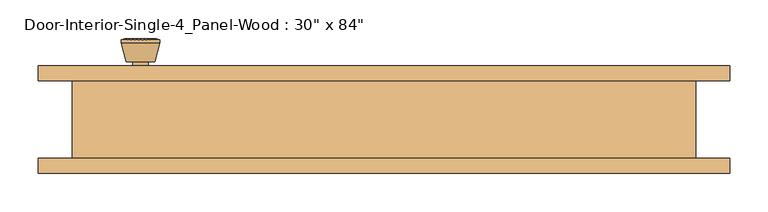
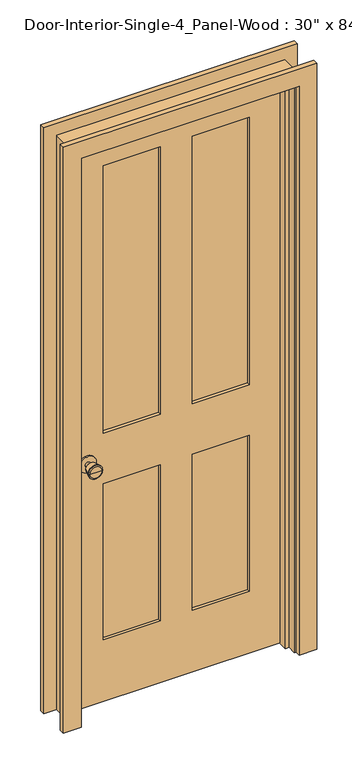
"""IFC4 building model written with IfcOpenShell, lengths in millimetres: door geometry."""

from ifc_helpers import new_model, si_unit, point, frame, frame_2d, origin, place, context, project, spatial, polyline, circle_curve, trimmed, segment, composite_curve, outline, extrude, faceted_brep, source, transform, mapped, element, save
from ifc_brep_helpers import plane_surface, cylinder_surface, revolved_surface, advanced_brep


def door_bd7b73b2(model_context):
    return source(origin(), model_context, "Body", "SolidModel", [
        advanced_brep(
        [(-317.5, 6.7, 914.4), (-307.5, 6.7, 914.4), (-327.5, 6.7, 914.4), (-297.0241324, -42.3, 914.4), (-317.5, -42.3, 914.4), (-337.9758676, -42.3, 914.4), (-292.5, -40.4721319, 914.4), (-342.5, -40.4721319, 914.4), (-292.5, -37.0084537, 914.4), (-342.5, -37.0084537, 914.4), (-298.863764, -12.3, 914.4), (-336.136236, -12.3, 914.4), (-307.5, -12.3, 914.4), (-327.5, -12.3, 914.4)],
        [
            (0, 1),
            (1, 2, circle_curve(frame((-317.5, 6.7, 914.4), z_axis=(0.0, 1.0, 0.0), x_axis=(-1.0, 0.0, 0.0)), 10.0)),
            (2, 0),
            (2, 1, circle_curve(frame((-317.5, 6.7, 914.4), z_axis=(0.0, 1.0, 0.0), x_axis=(-1.0, 0.0, 0.0)), 10.0)),
            (3, 4),
            (4, 5),
            (5, 3, circle_curve(frame((-317.5, -42.3, 914.4), z_axis=(0.0, -1.0, 0.0), x_axis=(-1.0, 0.0, 0.0)), 20.4758676)),
            (3, 5, circle_curve(frame((-317.5, -42.3, 914.4), z_axis=(0.0, -1.0, 0.0), x_axis=(-1.0, 0.0, 0.0)), 20.4758676)),
            (6, 3),
            (5, 7),
            (7, 6, circle_curve(frame((-317.5, -40.4721319, 914.4), z_axis=(0.0, -1.0, 0.0), x_axis=(-1.0, 0.0, 0.0)), 25.0)),
            (6, 7, circle_curve(frame((-317.5, -40.4721319, 914.4), z_axis=(0.0, -1.0, 0.0), x_axis=(-1.0, 0.0, 0.0)), 25.0)),
            (8, 6),
            (7, 9),
            (9, 8, circle_curve(frame((-317.5, -37.0084537, 914.4), z_axis=(0.0, -1.0, 0.0), x_axis=(-1.0, 0.0, 0.0)), 25.0)),
            (8, 9, circle_curve(frame((-317.5, -37.0084537, 914.4), z_axis=(0.0, -1.0, 0.0), x_axis=(-1.0, 0.0, 0.0)), 25.0)),
            (10, 8),
            (9, 11),
            (11, 10, circle_curve(frame((-317.5, -12.3, 914.4), z_axis=(0.0, -1.0, 0.0), x_axis=(-1.0, 0.0, 0.0)), 18.636236)),
            (10, 11, circle_curve(frame((-317.5, -12.3, 914.4), z_axis=(0.0, -1.0, 0.0), x_axis=(-1.0, 0.0, 0.0)), 18.636236)),
            (12, 10),
            (11, 13),
            (13, 12, circle_curve(frame((-317.5, -12.3, 914.4), z_axis=(0.0, -1.0, 0.0), x_axis=(-1.0, 0.0, 0.0)), 10.0)),
            (12, 13, circle_curve(frame((-317.5, -12.3, 914.4), z_axis=(0.0, -1.0, 0.0), x_axis=(-1.0, 0.0, 0.0)), 10.0)),
            (1, 12),
            (13, 2),
        ],
        [
            plane_surface(frame((-317.5, 6.7, 914.4), z_axis=(0.0, 1.0, 0.0), x_axis=(-1.0, 0.0, 0.0))),
            plane_surface(frame((-317.5, -42.3, 914.4), z_axis=(0.0, -1.0, 0.0), x_axis=(-1.0, 0.0, 0.0))),
            revolved_surface(polyline([(-337.9758676, -42.3, 914.4), (-342.5, -40.4721319, 914.4)]), (-317.5, 6.7, 914.4), (0.0, 1.0, 0.0)),
            cylinder_surface(frame((-317.5, 6.7, 914.4), z_axis=(0.0, 1.0, 0.0), x_axis=(-1.0, 0.0, 0.0)), 25.0),
            revolved_surface(polyline([(-342.5, -37.0084537, 914.4), (-336.136236, -12.3, 914.4)]), (-317.5, 6.7, 914.4), (0.0, 1.0, 0.0)),
            plane_surface(frame((-317.5, -12.3, 914.4), z_axis=(0.0, 1.0, 0.0), x_axis=(-1.0, 0.0, 0.0))),
            cylinder_surface(frame((-317.5, 6.7, 914.4), z_axis=(0.0, 1.0, 0.0), x_axis=(-1.0, 0.0, 0.0)), 10.0),
        ],
        [
            (0, [[1, 2, 3]]),
            (0, [[-3, 4, -1]]),
            (1, [[5, 6, 7]]),
            (1, [[-6, -5, 8]]),
            (2, [[9, -7, 10, 11]]),
            (2, [[-10, -8, -9, 12]]),
            (3, [[13, -11, 14, 15]]),
            (3, [[-14, -12, -13, 16]]),
            (4, [[17, -15, 18, 19]]),
            (4, [[-18, -16, -17, 20]]),
            (5, [[21, -19, 22, 23]]),
            (5, [[-22, -20, -21, 24]]),
            (6, [[25, -23, 26, -2]]),
            (6, [[-26, -24, -25, -4]]),
        ],
    ),
        extrude(outline(composite_curve([segment(trimmed(circle_curve(frame_2d((914.4, -317.5)), 30.0), [point((914.4, -347.5))], [point((914.4, -287.5))], False, "CARTESIAN"), True, "CONTINUOUS"), segment(trimmed(circle_curve(frame_2d((914.4, -317.5)), 30.0), [point((914.4, -287.5))], [point((914.4, -347.5))], False, "CARTESIAN"), True, "CONTINUOUS")], self_intersect=False)), frame((0.0, 6.7, 0.0), z_axis=(0.0, 1.0, 0.0), x_axis=(0.0, 0.0, 1.0)), (0.0, 0.0, 1.0), 6.0),
        advanced_brep(
        [(-317.5, 53.625, 914.4), (-327.5, 53.625, 914.4), (-307.5, 53.625, 914.4), (-297.0241324, 102.625, 914.4), (-337.9758676, 102.625, 914.4), (-317.5, 102.625, 914.4), (-292.5, 100.7971319, 914.4), (-342.5, 100.7971319, 914.4), (-292.5, 97.3334537, 914.4), (-342.5, 97.3334537, 914.4), (-298.863764, 72.625, 914.4), (-336.136236, 72.625, 914.4), (-307.5, 72.625, 914.4), (-327.5, 72.625, 914.4)],
        [
            (0, 1),
            (1, 2, circle_curve(frame((-317.5, 53.625, 914.4), z_axis=(0.0, -1.0, 0.0), x_axis=(-1.0, 0.0, 0.0)), 10.0)),
            (2, 0),
            (2, 1, circle_curve(frame((-317.5, 53.625, 914.4), z_axis=(0.0, -1.0, 0.0), x_axis=(-1.0, 0.0, 0.0)), 10.0)),
            (3, 4, circle_curve(frame((-317.5, 102.625, 914.4), z_axis=(0.0, 1.0, 0.0), x_axis=(-1.0, 0.0, 0.0)), 20.4758676)),
            (4, 5),
            (5, 3),
            (4, 3, circle_curve(frame((-317.5, 102.625, 914.4), z_axis=(0.0, 1.0, 0.0), x_axis=(-1.0, 0.0, 0.0)), 20.4758676)),
            (6, 7, circle_curve(frame((-317.5, 100.7971319, 914.4), z_axis=(0.0, 1.0, 0.0), x_axis=(-1.0, 0.0, 0.0)), 25.0)),
            (7, 4),
            (3, 6),
            (7, 6, circle_curve(frame((-317.5, 100.7971319, 914.4), z_axis=(0.0, 1.0, 0.0), x_axis=(-1.0, 0.0, 0.0)), 25.0)),
            (8, 9, circle_curve(frame((-317.5, 97.3334537, 914.4), z_axis=(0.0, 1.0, 0.0), x_axis=(-1.0, 0.0, 0.0)), 25.0)),
            (9, 7),
            (6, 8),
            (9, 8, circle_curve(frame((-317.5, 97.3334537, 914.4), z_axis=(0.0, 1.0, 0.0), x_axis=(-1.0, 0.0, 0.0)), 25.0)),
            (10, 11, circle_curve(frame((-317.5, 72.625, 914.4), z_axis=(0.0, 1.0, 0.0), x_axis=(-1.0, 0.0, 0.0)), 18.636236)),
            (11, 9),
            (8, 10),
            (11, 10, circle_curve(frame((-317.5, 72.625, 914.4), z_axis=(0.0, 1.0, 0.0), x_axis=(-1.0, 0.0, 0.0)), 18.636236)),
            (12, 13, circle_curve(frame((-317.5, 72.625, 914.4), z_axis=(0.0, 1.0, 0.0), x_axis=(-1.0, 0.0, 0.0)), 10.0)),
            (13, 11),
            (10, 12),
            (13, 12, circle_curve(frame((-317.5, 72.625, 914.4), z_axis=(0.0, 1.0, 0.0), x_axis=(-1.0, 0.0, 0.0)), 10.0)),
            (1, 13),
            (12, 2),
        ],
        [
            plane_surface(frame((-317.5, 53.625, 914.4), z_axis=(0.0, -1.0, 0.0), x_axis=(-1.0, 0.0, 0.0))),
            plane_surface(frame((-317.5, 102.625, 914.4), z_axis=(0.0, 1.0, 0.0), x_axis=(-1.0, 0.0, 0.0))),
            revolved_surface(polyline([(-337.9758676, 102.625, 914.4), (-342.5, 100.7971319, 914.4)]), (-317.5, 53.625, 914.4), (0.0, -1.0, 0.0)),
            cylinder_surface(frame((-317.5, 53.625, 914.4), z_axis=(0.0, -1.0, 0.0), x_axis=(-1.0, 0.0, 0.0)), 25.0),
            revolved_surface(polyline([(-342.5, 97.3334537, 914.4), (-336.136236, 72.625, 914.4)]), (-317.5, 53.625, 914.4), (0.0, -1.0, 0.0)),
            plane_surface(frame((-317.5, 72.625, 914.4), z_axis=(0.0, -1.0, 0.0), x_axis=(-1.0, 0.0, 0.0))),
            cylinder_surface(frame((-317.5, 53.625, 914.4), z_axis=(0.0, -1.0, 0.0), x_axis=(-1.0, 0.0, 0.0)), 10.0),
        ],
        [
            (0, [[1, 2, 3]]),
            (0, [[-3, 4, -1]]),
            (1, [[5, 6, 7]]),
            (1, [[8, -7, -6]]),
            (2, [[9, 10, -5, 11]]),
            (2, [[12, -11, -8, -10]]),
            (3, [[13, 14, -9, 15]]),
            (3, [[16, -15, -12, -14]]),
            (4, [[17, 18, -13, 19]]),
            (4, [[20, -19, -16, -18]]),
            (5, [[21, 22, -17, 23]]),
            (5, [[24, -23, -20, -22]]),
            (6, [[-2, 25, -21, 26]]),
            (6, [[-4, -26, -24, -25]]),
        ],
    ),
        extrude(outline(composite_curve([segment(trimmed(circle_curve(frame_2d((914.4, -317.5)), 30.0), [point((914.4, -347.5))], [point((914.4, -287.5))], False, "CARTESIAN"), True, "CONTINUOUS"), segment(trimmed(circle_curve(frame_2d((914.4, -317.5)), 30.0), [point((914.4, -287.5))], [point((914.4, -347.5))], False, "CARTESIAN"), True, "CONTINUOUS")], self_intersect=False)), frame((0.0, 47.625, 0.0), z_axis=(0.0, 1.0, 0.0), x_axis=(0.0, 0.0, 1.0)), (0.0, 0.0, 1.0), 6.0),
        extrude(outline(polyline([(260.35, 24.3416667), (57.15, 24.3416667), (57.15, 35.9833333), (260.35, 35.9833333), (260.35, 24.3416667)])), frame((0.0, 0.0, 1009.65), z_axis=(0.0, 0.0, 1.0), x_axis=(1.0, 0.0, 0.0)), (0.0, 0.0, 1.0), 1004.8875),
        extrude(outline(polyline([(-57.15, 24.3416667), (-260.35, 24.3416667), (-260.35, 35.9833333), (-57.15, 35.9833333), (-57.15, 24.3416667)])), frame((0.0, 0.0, 1009.65), z_axis=(0.0, 0.0, 1.0), x_axis=(1.0, 0.0, 0.0)), (0.0, 0.0, 1.0), 1004.8875),
        extrude(outline(polyline([(260.35, 24.3416667), (57.15, 24.3416667), (57.15, 35.9833333), (260.35, 35.9833333), (260.35, 24.3416667)])), frame((0.0, 0.0, 231.775), z_axis=(0.0, 0.0, 1.0), x_axis=(1.0, 0.0, 0.0)), (0.0, 0.0, 1.0), 587.375),
        extrude(outline(polyline([(-57.15, 24.3416667), (-260.35, 24.3416667), (-260.35, 35.9833333), (-57.15, 35.9833333), (-57.15, 24.3416667)])), frame((0.0, 0.0, 231.775), z_axis=(0.0, 0.0, 1.0), x_axis=(1.0, 0.0, 0.0)), (0.0, 0.0, 1.0), 587.375),
        extrude(outline(polyline([(2133.6, -381.0), (0.0, -381.0), (0.0, 381.0), (2133.6, 381.0), (2133.6, -381.0)]), holes=[polyline([(2014.5375, 57.15), (2014.5375, 260.35), (1009.65, 260.35), (1009.65, 57.15), (2014.5375, 57.15)]), polyline([(1009.65, -57.15), (1009.65, -260.35), (2014.5375, -260.35), (2014.5375, -57.15), (1009.65, -57.15)]), polyline([(819.15, 57.15), (819.15, 260.35), (231.775, 260.35), (231.775, 57.15), (819.15, 57.15)]), polyline([(231.775, -57.15), (231.775, -260.35), (819.15, -260.35), (819.15, -57.15), (231.775, -57.15)])]), frame((0.0, 12.7, 0.0), z_axis=(0.0, 1.0, 0.0), x_axis=(0.0, 0.0, 1.0)), (0.0, 0.0, 1.0), 34.925),
        faceted_brep([(406.4, 47.625, 0.0), (406.4, -53.975, 0.0), (381.0, -53.975, 0.0), (381.0, -22.225, 0.0), (368.3, -22.225, 0.0), (368.3, 12.7, 0.0), (381.0, 12.7, 0.0), (381.0, 47.625, 0.0), (406.4, 47.625, 2159.0), (406.4, -53.975, 2159.0), (-406.4, -53.975, 2159.0), (-406.4, -53.975, 0.0), (-381.0, -53.975, 0.0), (-381.0, -53.975, 2133.6), (381.0, -53.975, 2133.6), (381.0, -22.225, 2133.6), (-381.0, -22.225, 2133.6), (-381.0, -22.225, 0.0), (-368.3, -22.225, 0.0), (-368.3, -22.225, 2120.9), (368.3, -22.225, 2120.9), (368.3, 12.7, 2120.9), (-368.3, 12.7, 2120.9), (-368.3, 12.7, 0.0), (-381.0, 12.7, 0.0), (-381.0, 12.7, 2133.6), (381.0, 12.7, 2133.6), (381.0, 47.625, 2133.6), (-381.0, 47.625, 2133.6), (-381.0, 47.625, 0.0), (-406.4, 47.625, 0.0), (-406.4, 47.625, 2159.0)], [[[0, 1, 2, 3, 4, 5, 6, 7]], [[1, 0, 8, 9]], [[2, 1, 9, 10, 11, 12, 13, 14]], [[3, 2, 14, 15]], [[4, 3, 15, 16, 17, 18, 19, 20]], [[5, 4, 20, 21]], [[6, 5, 21, 22, 23, 24, 25, 26]], [[7, 6, 26, 27]], [[0, 7, 27, 28, 29, 30, 31, 8]], [[9, 8, 31, 10]], [[15, 14, 13, 16]], [[21, 20, 19, 22]], [[27, 26, 25, 28]], [[30, 29, 24, 23, 18, 17, 12, 11]], [[10, 31, 30, 11]], [[16, 13, 12, 17]], [[22, 19, 18, 23]], [[28, 25, 24, 29]]]),
        extrude(outline(polyline([(0.0, 387.35), (0.0, 450.85), (2203.45, 450.85), (2203.45, -450.85), (0.0, -450.85), (0.0, -387.35), (2139.95, -387.35), (2139.95, 387.35), (0.0, 387.35)])), frame((0.0, -73.025, 0.0), z_axis=(0.0, 1.0, 0.0), x_axis=(0.0, 0.0, 1.0)), (0.0, 0.0, 1.0), 19.05),
        extrude(outline(polyline([(0.0, 387.35), (0.0, 450.85), (2203.45, 450.85), (2203.45, -450.85), (0.0, -450.85), (0.0, -387.35), (2139.95, -387.35), (2139.95, 387.35), (0.0, 387.35)])), frame((0.0, 47.625, 0.0), z_axis=(0.0, 1.0, 0.0), x_axis=(0.0, 0.0, 1.0)), (0.0, 0.0, 1.0), 19.05),
    ])


if __name__ == "__main__":
    model = new_model("IFC4")
    model_context = context("Model", 3, world=origin())
    ifc_project = project(units=[si_unit("LENGTHUNIT", "METRE", prefix="MILLI")], contexts=[model_context])
    site = spatial("IfcSite", under=ifc_project)
    building = spatial("IfcBuilding", under=site)
    placement = place(None, origin())
    door_shape = door_bd7b73b2(model_context)
    element("IfcDoor", 1, ObjectType="Door-Interior-Single-4_Panel-Wood : 30\" x 84\"", at=placement, inside=building, context=model_context, shape_type="MappedRepresentation", body=[
        mapped(door_shape, transform((0.0, 0.0, 0.0), x_axis=(1.0, 0.0, 0.0), y_axis=(0.0, 1.0, 0.0), z_axis=(0.0, 0.0, 1.0))),
    ])
    save(model, "model.ifc")

# Revit data of these elements
# Type "Door-Interior-Single-4_Panel-Wood : 30\" x 84\""
#   Type Mark = "9"
#   Assembly Code = "C1020300"
#   Analytic Construction = "Wooden"
#   Top Rail = 0' - 4 11/16"
#   Thickness = 0' - 1 3/8"
#   Thermal Resistance (R) = 2.5876 (h·ft²·°F)/BTU
#   Swing Angle [instance default] = 90.00°
#   Stiles = 0' - 4 3/4"
#   Rough Width = 2' - 8"
#   Rough Height = 7' - 1"
#   Mullion = 0' - 4 1/2"
#   Lock Rail = 0' - 7 1/2"
#   Height = 7' - 0"
#   Width = 2' - 6"
#   Heat Transfer Coefficient (U) = 0.3865 BTU/(h·ft²·°F)
#   Bottom Rail = 0' - 9 1/8"
#   Trim Material = Cherry
#   Panel Material = Cherry
#   Frame Material = Cherry
#   Door Handle Material = Aluminum
#   Visual Light Transmittance = 0
#   Solar Heat Gain Coefficient = 0
#   Wall Closure = (empty or 0)
#   Function = (empty or 0)
# Element 1 (IfcDoor, "Door-Interior-Single-4_Panel-Wood : 30\" x 84\"")
#   Materials on its faces: "Cherry", "Aluminum"
# Materials
#   "Cherry": class "Wood", colour RGB 226 177 128, transparency 0, Description = "Prunus Serotina", Cost = 0
#   "Aluminum": class "Metal", colour RGB 247 247 247, transparency 0, Description = "Aluminum 6061", Cost = 0
